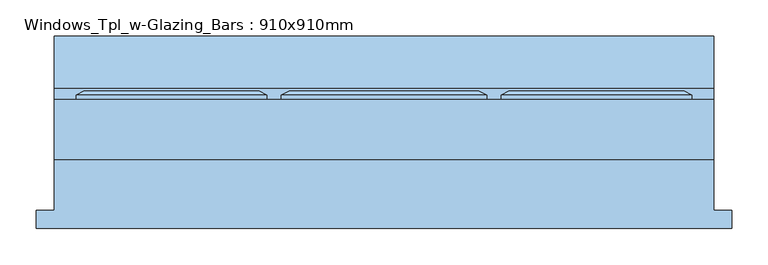
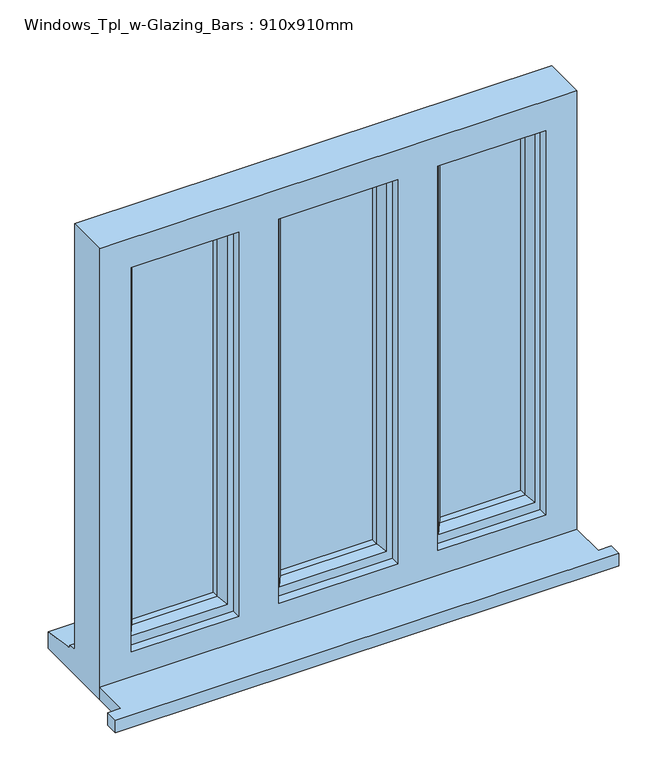
"""IFC4 building model written with IfcOpenShell, lengths in millimetres: window geometry, Windows_Tpl_w-Glazing_Bars : 910x910mm."""

from ifc_helpers import new_model, si_unit, frame, origin, place, context, project, spatial, polyline, outline, extrude, faceted_brep, source, transform, mapped, element, save


def windows_tpl_w_glazing_bars_910x910mm_9d987a72(model_context):
    return source(origin(), model_context, "Body", "SolidModel", [
        extrude(outline(polyline([(-716.6666667, -118.1434322), (-716.6666667, -93.1434322), (-691.6666667, -93.1434322), (-691.6666667, -22.9434322), (218.3333333, -22.9434322), (218.3333333, -93.1434322), (243.3333333, -93.1434322), (243.3333333, -118.1434322), (-716.6666667, -118.1434322)])), frame((0.0, 0.0, 1200.0), z_axis=(0.0, 0.0, 1.0), x_axis=(1.0, 0.0, 0.0)), (0.0, 0.0, 1.0), 25.0),
        faceted_brep([(-75.0, 60.0565678, 2080.0), (-75.0, 65.8300705, 2080.0), (-75.0, 65.8300705, 1253.0), (-75.0, 60.0565678, 1253.0), (-65.0, -4.9434322, 2070.0), (-65.0, 60.0565678, 2070.0), (-65.0, 60.0565678, 1263.0), (-65.0, -4.9434322, 1263.0), (-25.0, 9.5494677, 2030.0), (-35.1480377, -4.9434322, 2040.1480377), (-35.1480377, -4.9434322, 1292.8519623), (-25.0, 9.5494677, 1303.0), (-25.0, 24.0565678, 2030.0), (-25.0, 24.0565678, 1303.0), (-35.0, 48.0565678, 2040.0), (-35.0, 24.0565678, 2040.0), (-35.0, 24.0565678, 1293.0), (-35.0, 48.0565678, 1293.0), (-25.0, 65.8300705, 2030.0), (-25.0, 48.0565678, 2030.0), (-25.0, 48.0565678, 1303.0), (-25.0, 65.8300705, 1303.0), (-42.4457548, 71.6035732, 2047.4457548), (-42.4457548, 71.6035732, 1285.5542452), (-64.2153903, 71.6035732, 2069.2153903), (-64.2153903, 71.6035732, 1263.7846097), (188.3333333, 65.8300705, 1253.0), (188.3333333, 60.0565678, 1253.0), (178.3333333, 60.0565678, 1263.0), (178.3333333, -4.9434322, 1263.0), (148.4813711, -4.9434322, 1292.8519623), (138.3333333, 9.5494677, 1303.0), (138.3333333, 24.0565678, 1303.0), (148.3333333, 24.0565678, 1293.0), (148.3333333, 48.0565678, 1293.0), (138.3333333, 48.0565678, 1303.0), (138.3333333, 65.8300705, 1303.0), (155.7790881, 71.6035732, 1285.5542452), (177.5487236, 71.6035732, 1263.7846097), (188.3333333, 65.8300705, 2080.0), (188.3333333, 60.0565678, 2080.0), (178.3333333, 60.0565678, 2070.0), (178.3333333, -4.9434322, 2070.0), (148.4813711, -4.9434322, 2040.1480377), (138.3333333, 9.5494677, 2030.0), (138.3333333, 24.0565678, 2030.0), (148.3333333, 24.0565678, 2040.0), (148.3333333, 48.0565678, 2040.0), (138.3333333, 48.0565678, 2030.0), (138.3333333, 65.8300705, 2030.0), (155.7790881, 71.6035732, 2047.4457548), (177.5487236, 71.6035732, 2069.2153903)], [[[0, 1, 2, 3]], [[4, 5, 6, 7]], [[8, 9, 10, 11]], [[12, 8, 11, 13]], [[14, 15, 16, 17]], [[18, 19, 20, 21]], [[22, 18, 21, 23]], [[1, 24, 25, 2]], [[3, 2, 26, 27]], [[7, 6, 28, 29]], [[11, 10, 30, 31]], [[13, 11, 31, 32]], [[17, 16, 33, 34]], [[21, 20, 35, 36]], [[23, 21, 36, 37]], [[2, 25, 38, 26]], [[27, 26, 39, 40]], [[29, 28, 41, 42]], [[31, 30, 43, 44]], [[32, 31, 44, 45]], [[34, 33, 46, 47]], [[36, 35, 48, 49]], [[37, 36, 49, 50]], [[26, 38, 51, 39]], [[40, 39, 1, 0]], [[3, 27, 40, 0], [5, 41, 28, 6]], [[42, 41, 5, 4]], [[7, 29, 42, 4], [9, 43, 30, 10]], [[44, 43, 9, 8]], [[45, 44, 8, 12]], [[15, 46, 33, 16], [13, 32, 45, 12]], [[47, 46, 15, 14]], [[17, 34, 47, 14], [19, 48, 35, 20]], [[49, 48, 19, 18]], [[50, 49, 18, 22]], [[24, 51, 38, 25], [23, 37, 50, 22]], [[39, 51, 24, 1]]]),
        extrude(outline(polyline([(148.3333333, 24.0565678), (-35.1480377, 24.0565678), (-35.1480377, 48.0565678), (148.3333333, 48.0565678), (148.3333333, 24.0565678)])), frame((0.0, 0.0, 1293.0), z_axis=(0.0, 0.0, 1.0), x_axis=(1.0, 0.0, 0.0)), (0.0, 0.0, 1.0), 747.0),
        extrude(outline(polyline([(-135.0, 24.0565678), (-338.3333333, 24.0565678), (-338.3333333, 48.0565678), (-135.0, 48.0565678), (-135.0, 24.0565678)])), frame((0.0, 0.0, 1293.0), z_axis=(0.0, 0.0, 1.0), x_axis=(1.0, 0.0, 0.0)), (0.0, 0.0, 1.0), 747.0),
        extrude(outline(polyline([(-438.3333333, 24.0565678), (-621.6666667, 24.0565678), (-621.6666667, 48.0565678), (-438.3333333, 48.0565678), (-438.3333333, 24.0565678)])), frame((0.0, 0.0, 1293.0), z_axis=(0.0, 0.0, 1.0), x_axis=(1.0, 0.0, 0.0)), (0.0, 0.0, 1.0), 747.0),
        faceted_brep([(-398.3333333, 60.0565678, 2080.0), (-398.3333333, 65.8300705, 2080.0), (-661.6666667, 65.8300705, 2080.0), (-661.6666667, 60.0565678, 2080.0), (-408.3333333, -4.9434322, 2070.0), (-408.3333333, 60.0565678, 2070.0), (-651.6666667, 60.0565678, 2070.0), (-651.6666667, -4.9434322, 2070.0), (-448.3333333, 9.5494677, 2030.0), (-438.1852956, -4.9434322, 2040.1480377), (-621.8147044, -4.9434322, 2040.1480377), (-611.6666667, 9.5494677, 2030.0), (-448.3333333, 24.0565678, 2030.0), (-611.6666667, 24.0565678, 2030.0), (-438.3333333, 48.0565678, 2040.0), (-438.3333333, 24.0565678, 2040.0), (-621.6666667, 24.0565678, 2040.0), (-621.6666667, 48.0565678, 2040.0), (-448.3333333, 65.8300705, 2030.0), (-448.3333333, 48.0565678, 2030.0), (-611.6666667, 48.0565678, 2030.0), (-611.6666667, 65.8300705, 2030.0), (-430.8875785, 71.6035732, 2047.4457548), (-629.1124215, 71.6035732, 2047.4457548), (-409.117943, 71.6035732, 2069.2153903), (-650.882057, 71.6035732, 2069.2153903), (-661.6666667, 65.8300705, 1253.0), (-661.6666667, 60.0565678, 1253.0), (-651.6666667, 60.0565678, 1263.0), (-651.6666667, -4.9434322, 1263.0), (-621.8147044, -4.9434322, 1292.8519623), (-611.6666667, 9.5494677, 1303.0), (-611.6666667, 24.0565678, 1303.0), (-621.6666667, 24.0565678, 1293.0), (-621.6666667, 48.0565678, 1293.0), (-611.6666667, 48.0565678, 1303.0), (-611.6666667, 65.8300705, 1303.0), (-629.1124215, 71.6035732, 1285.5542452), (-650.882057, 71.6035732, 1263.7846097), (-398.3333333, 65.8300705, 1253.0), (-398.3333333, 60.0565678, 1253.0), (-408.3333333, 60.0565678, 1263.0), (-408.3333333, -4.9434322, 1263.0), (-438.1852956, -4.9434322, 1292.8519623), (-448.3333333, 9.5494677, 1303.0), (-448.3333333, 24.0565678, 1303.0), (-438.3333333, 24.0565678, 1293.0), (-438.3333333, 48.0565678, 1293.0), (-448.3333333, 48.0565678, 1303.0), (-448.3333333, 65.8300705, 1303.0), (-430.8875785, 71.6035732, 1285.5542452), (-409.117943, 71.6035732, 1263.7846097)], [[[0, 1, 2, 3]], [[4, 5, 6, 7]], [[8, 9, 10, 11]], [[12, 8, 11, 13]], [[14, 15, 16, 17]], [[18, 19, 20, 21]], [[22, 18, 21, 23]], [[1, 24, 25, 2]], [[3, 2, 26, 27]], [[7, 6, 28, 29]], [[11, 10, 30, 31]], [[13, 11, 31, 32]], [[17, 16, 33, 34]], [[21, 20, 35, 36]], [[23, 21, 36, 37]], [[2, 25, 38, 26]], [[27, 26, 39, 40]], [[0, 3, 27, 40], [41, 28, 6, 5]], [[29, 28, 41, 42]], [[4, 7, 29, 42], [43, 30, 10, 9]], [[31, 30, 43, 44]], [[32, 31, 44, 45]], [[46, 33, 16, 15], [12, 13, 32, 45]], [[34, 33, 46, 47]], [[14, 17, 34, 47], [48, 35, 20, 19]], [[36, 35, 48, 49]], [[37, 36, 49, 50]], [[51, 38, 25, 24], [22, 23, 37, 50]], [[26, 38, 51, 39]], [[40, 39, 1, 0]], [[42, 41, 5, 4]], [[44, 43, 9, 8]], [[45, 44, 8, 12]], [[47, 46, 15, 14]], [[49, 48, 19, 18]], [[50, 49, 18, 22]], [[39, 51, 24, 1]]]),
        extrude(outline(polyline([(-35.0, 40.0565678), (148.3333333, 40.0565678), (148.3333333, 32.0565678), (-35.0, 32.0565678), (-35.0, 40.0565678)])), frame((0.0, 0.0, 1656.5), z_axis=(0.0, 0.0, 1.0), x_axis=(1.0, 0.0, 0.0)), (0.0, 0.0, 1.0), 20.0),
        extrude(outline(polyline([(-621.6666667, 40.0565678), (-438.3333333, 40.0565678), (-438.3333333, 32.0565678), (-621.6666667, 32.0565678), (-621.6666667, 40.0565678)])), frame((0.0, 0.0, 1656.5), z_axis=(0.0, 0.0, 1.0), x_axis=(1.0, 0.0, 0.0)), (0.0, 0.0, 1.0), 20.0),
        extrude(outline(polyline([(-35.0, 40.0565678), (148.3333333, 40.0565678), (148.3333333, 32.0565678), (-35.0, 32.0565678), (-35.0, 40.0565678)])), frame((0.0, 0.0, 1838.25), z_axis=(0.0, 0.0, 1.0), x_axis=(1.0, 0.0, 0.0)), (0.0, 0.0, 1.0), 20.0),
        extrude(outline(polyline([(-35.0, 40.0565678), (148.3333333, 40.0565678), (148.3333333, 32.0565678), (-35.0, 32.0565678), (-35.0, 40.0565678)])), frame((0.0, 0.0, 1474.75), z_axis=(0.0, 0.0, 1.0), x_axis=(1.0, 0.0, 0.0)), (0.0, 0.0, 1.0), 20.0),
        extrude(outline(polyline([(-621.6666667, 40.0565678), (-438.3333333, 40.0565678), (-438.3333333, 32.0565678), (-621.6666667, 32.0565678), (-621.6666667, 40.0565678)])), frame((0.0, 0.0, 1838.25), z_axis=(0.0, 0.0, 1.0), x_axis=(1.0, 0.0, 0.0)), (0.0, 0.0, 1.0), 20.0),
        extrude(outline(polyline([(-621.6666667, 40.0565678), (-438.3333333, 40.0565678), (-438.3333333, 32.0565678), (-621.6666667, 32.0565678), (-621.6666667, 40.0565678)])), frame((0.0, 0.0, 1474.75), z_axis=(0.0, 0.0, 1.0), x_axis=(1.0, 0.0, 0.0)), (0.0, 0.0, 1.0), 20.0),
        extrude(outline(polyline([(-338.3333333, 40.0565678), (-135.0, 40.0565678), (-135.0, 32.0565678), (-338.3333333, 32.0565678), (-338.3333333, 40.0565678)])), frame((0.0, 0.0, 1656.5), z_axis=(0.0, 0.0, 1.0), x_axis=(1.0, 0.0, 0.0)), (0.0, 0.0, 1.0), 20.0),
        extrude(outline(polyline([(-338.3333333, 40.0565678), (-135.0, 40.0565678), (-135.0, 32.0565678), (-338.3333333, 32.0565678), (-338.3333333, 40.0565678)])), frame((0.0, 0.0, 1838.25), z_axis=(0.0, 0.0, 1.0), x_axis=(1.0, 0.0, 0.0)), (0.0, 0.0, 1.0), 20.0),
        extrude(outline(polyline([(-338.3333333, 40.0565678), (-135.0, 40.0565678), (-135.0, 32.0565678), (-338.3333333, 32.0565678), (-338.3333333, 40.0565678)])), frame((0.0, 0.0, 1474.75), z_axis=(0.0, 0.0, 1.0), x_axis=(1.0, 0.0, 0.0)), (0.0, 0.0, 1.0), 20.0),
        faceted_brep([(218.3333333, -22.9434322, 2110.0), (-691.6666667, -22.9434322, 2110.0), (-691.6666667, -22.9434322, 1200.0), (218.3333333, -22.9434322, 1200.0), (158.3333333, -22.9434322, 2050.0), (158.3333333, -22.9434322, 1275.0), (-47.0, -22.9434322, 1275.0), (-47.0, -22.9434322, 2050.0), (-123.0, -22.9434322, 2050.0), (-123.0, -22.9434322, 1275.0), (-350.3333333, -22.9434322, 1275.0), (-350.3333333, -22.9434322, 2050.0), (-426.3333333, -22.9434322, 2050.0), (-426.3333333, -22.9434322, 1275.0), (-631.6666667, -22.9434322, 1275.0), (-631.6666667, -22.9434322, 2050.0), (-691.6666667, 60.0565678, 2110.0), (-691.6666667, 60.0565678, 1251.0), (-691.6666667, 75.0565678, 1249.68767), (-691.6666667, 75.0565678, 1244.7449676), (-691.6666667, 147.5565678, 1233.8088847), (-691.6666667, 147.5565678, 1200.0), (218.3333333, 60.0565678, 2110.0), (218.3333333, 60.0565678, 1251.0), (-651.6666667, 60.0565678, 2070.0), (-651.6666667, 60.0565678, 1263.0), (-408.3333333, 60.0565678, 1263.0), (-408.3333333, 60.0565678, 2070.0), (-368.3333333, 60.0565678, 2070.0), (-368.3333333, 60.0565678, 1263.0), (-105.0, 60.0565678, 1263.0), (-105.0, 60.0565678, 2070.0), (-65.0, 60.0565678, 2070.0), (-65.0, 60.0565678, 1263.0), (178.3333333, 60.0565678, 1263.0), (178.3333333, 60.0565678, 2070.0), (-651.6666667, -4.9434322, 2070.0), (-651.6666667, -4.9434322, 1263.0), (-368.3333333, -4.9434322, 2070.0), (-105.0, -4.9434322, 2070.0), (-105.0, -4.9434322, 1263.0), (-368.3333333, -4.9434322, 1263.0), (-123.0, -4.9434322, 2050.0), (-350.3333333, -4.9434322, 2050.0), (-350.3333333, -4.9434322, 1275.0), (-123.0, -4.9434322, 1275.0), (-65.0, -4.9434322, 2070.0), (178.3333333, -4.9434322, 2070.0), (178.3333333, -4.9434322, 1263.0), (-65.0, -4.9434322, 1263.0), (158.3333333, -4.9434322, 2050.0), (-47.0, -4.9434322, 2050.0), (-47.0, -4.9434322, 1275.0), (158.3333333, -4.9434322, 1275.0), (-408.3333333, -4.9434322, 2070.0), (-408.3333333, -4.9434322, 1263.0), (-426.3333333, -4.9434322, 2050.0), (-631.6666667, -4.9434322, 2050.0), (-631.6666667, -4.9434322, 1275.0), (-426.3333333, -4.9434322, 1275.0), (218.3333333, 147.5565678, 1200.0), (218.3333333, 147.5565678, 1233.8088847), (218.3333333, 75.0565678, 1244.7449676), (218.3333333, 75.0565678, 1249.68767)], [[[0, 1, 2, 3], [4, 5, 6, 7], [8, 9, 10, 11], [12, 13, 14, 15]], [[2, 1, 16, 17, 18, 19, 20, 21]], [[17, 16, 22, 23], [24, 25, 26, 27], [28, 29, 30, 31], [32, 33, 34, 35]], [[25, 24, 36, 37]], [[38, 39, 40, 41], [42, 43, 44, 45]], [[46, 47, 48, 49], [50, 51, 52, 53]], [[36, 54, 55, 37], [56, 57, 58, 59]], [[57, 15, 14, 58]], [[1, 0, 22, 16]], [[36, 24, 27, 54]], [[35, 47, 46, 32]], [[38, 28, 31, 39]], [[15, 57, 56, 12]], [[50, 4, 7, 51]], [[11, 43, 42, 8]], [[23, 22, 0, 3, 60, 61, 62, 63]], [[35, 34, 48, 47]], [[4, 50, 53, 5]], [[43, 11, 10, 44]], [[12, 56, 59, 13]], [[27, 26, 55, 54]], [[29, 28, 38, 41]], [[31, 30, 40, 39]], [[33, 32, 46, 49]], [[51, 7, 6, 52]], [[8, 42, 45, 9]], [[60, 3, 2, 21]], [[61, 60, 21, 20]], [[62, 61, 20, 19]], [[63, 62, 19, 18]], [[23, 63, 18, 17]], [[26, 25, 37, 55]], [[34, 33, 49, 48]], [[41, 40, 30, 29]], [[6, 5, 53, 52]], [[45, 44, 10, 9]], [[59, 58, 14, 13]]]),
        faceted_brep([(-378.3333333, 60.0565678, 2080.0), (-378.3333333, 65.8300705, 2080.0), (-378.3333333, 65.8300705, 1253.0), (-378.3333333, 60.0565678, 1253.0), (-368.3333333, -4.9434322, 2070.0), (-368.3333333, 60.0565678, 2070.0), (-368.3333333, 60.0565678, 1263.0), (-368.3333333, -4.9434322, 1263.0), (-328.3333333, 9.5494677, 2030.0), (-338.4813711, -4.9434322, 2040.1480377), (-338.4813711, -4.9434322, 1292.8519623), (-328.3333333, 9.5494677, 1303.0), (-328.3333333, 24.0565678, 2030.0), (-328.3333333, 24.0565678, 1303.0), (-338.3333333, 48.0565678, 2040.0), (-338.3333333, 24.0565678, 2040.0), (-338.3333333, 24.0565678, 1293.0), (-338.3333333, 48.0565678, 1293.0), (-328.3333333, 65.8300705, 2030.0), (-328.3333333, 48.0565678, 2030.0), (-328.3333333, 48.0565678, 1303.0), (-328.3333333, 65.8300705, 1303.0), (-345.7790881, 71.6035732, 2047.4457548), (-345.7790881, 71.6035732, 1285.5542452), (-367.5487236, 71.6035732, 2069.2153903), (-367.5487236, 71.6035732, 1263.7846097), (-95.0, 65.8300705, 1253.0), (-95.0, 60.0565678, 1253.0), (-105.0, 60.0565678, 1263.0), (-105.0, -4.9434322, 1263.0), (-134.8519623, -4.9434322, 1292.8519623), (-145.0, 9.5494677, 1303.0), (-145.0, 24.0565678, 1303.0), (-135.0, 24.0565678, 1293.0), (-135.0, 48.0565678, 1293.0), (-145.0, 48.0565678, 1303.0), (-145.0, 65.8300705, 1303.0), (-127.5542452, 71.6035732, 1285.5542452), (-105.7846097, 71.6035732, 1263.7846097), (-95.0, 65.8300705, 2080.0), (-95.0, 60.0565678, 2080.0), (-105.0, 60.0565678, 2070.0), (-105.0, -4.9434322, 2070.0), (-134.8519623, -4.9434322, 2040.1480377), (-145.0, 9.5494677, 2030.0), (-145.0, 24.0565678, 2030.0), (-135.0, 24.0565678, 2040.0), (-135.0, 48.0565678, 2040.0), (-145.0, 48.0565678, 2030.0), (-145.0, 65.8300705, 2030.0), (-127.5542452, 71.6035732, 2047.4457548), (-105.7846097, 71.6035732, 2069.2153903)], [[[0, 1, 2, 3]], [[4, 5, 6, 7]], [[8, 9, 10, 11]], [[12, 8, 11, 13]], [[14, 15, 16, 17]], [[18, 19, 20, 21]], [[22, 18, 21, 23]], [[1, 24, 25, 2]], [[3, 2, 26, 27]], [[7, 6, 28, 29]], [[11, 10, 30, 31]], [[13, 11, 31, 32]], [[17, 16, 33, 34]], [[21, 20, 35, 36]], [[23, 21, 36, 37]], [[2, 25, 38, 26]], [[27, 26, 39, 40]], [[29, 28, 41, 42]], [[31, 30, 43, 44]], [[32, 31, 44, 45]], [[34, 33, 46, 47]], [[36, 35, 48, 49]], [[37, 36, 49, 50]], [[26, 38, 51, 39]], [[40, 39, 1, 0]], [[3, 27, 40, 0], [5, 41, 28, 6]], [[42, 41, 5, 4]], [[7, 29, 42, 4], [9, 43, 30, 10]], [[44, 43, 9, 8]], [[45, 44, 8, 12]], [[15, 46, 33, 16], [13, 32, 45, 12]], [[47, 46, 15, 14]], [[17, 34, 47, 14], [19, 48, 35, 20]], [[49, 48, 19, 18]], [[50, 49, 18, 22]], [[24, 51, 38, 25], [23, 37, 50, 22]], [[39, 51, 24, 1]]]),
    ])


if __name__ == "__main__":
    model = new_model("IFC4")
    model_context = context("Model", 3, world=origin())
    ifc_project = project(units=[si_unit("LENGTHUNIT", "METRE", prefix="MILLI")], contexts=[model_context])
    site = spatial("IfcSite", under=ifc_project)
    building = spatial("IfcBuilding", under=site)
    placement = place(None, origin())
    windows_tpl_w_glazing_bars_910x910mm_shape = windows_tpl_w_glazing_bars_910x910mm_9d987a72(model_context)
    element("IfcWindow", 1, ObjectType="Windows_Tpl_w-Glazing_Bars : 910x910mm", at=placement, inside=building, context=model_context, shape_type="MappedRepresentation", body=[
        mapped(windows_tpl_w_glazing_bars_910x910mm_shape, transform((0.0, 0.0, 0.0), x_axis=(1.0, 0.0, 0.0), y_axis=(0.0, 1.0, 0.0), z_axis=(0.0, 0.0, 1.0))),
    ])
    save(model, "model.ifc")

# Revit data of these elements
# Type "Windows_Tpl_w-Glazing_Bars : 910x910mm"
#   Type Mark = "18"
#   Operation = "TriplePanelVertical"
#   Construction Type Id = "GSP4R"
#   Manufacturer = "Revit"
#   Keynote = "L10"
#   Analytic Construction = "1/8 in Pilkington single glazing"
#   Length 1 = 24 mm
#   Wrap Layers (Ext) from Ext = 102.5 mm
#   Wrap Layers (Int) from Ext = 177.5 mm
#   Window Board Projection = 25 mm
#   Window Board Extension = 25 mm
#   Visual Light Transmittance = 0.9
#   Solar Heat Gain Coefficient = 0.78
#   Rough Width = 910 mm
#   Rough Height = 910 mm
#   Height = 910 mm
#   Width = 910 mm
#   Heat Transfer Coefficient (U) = 0.6496 BTU/(h·ft²·°F)
#   Glazing Thickness = 24 mm
#   Glazing Bar Thickness = 20 mm
#   FrameOffset - External = 50 mm
#   Frame Depth = 65 mm
#   Default Head Height = 2110 mm
#   Cill Depth = 87.5 mm
#   Cavity Closer Width = 50 mm
#   Cavity Closer Offset from Ext = 102.5 mm
#   Cavity Closer Depth = 85 mm
#   Vis - Glazing Bars = yes
#   Vis - Cavity Closers = yes
#   Define Thermal Properties by = 1
#   Material Trim = Window Frame
#   Material Glazing Bars = Window Frame
#   Material Glass = Glass
#   Material Frame = Window Frame
#   Wall Closure = (empty or 0)
# Element 1 (IfcWindow, "Windows_Tpl_w-Glazing_Bars : 910x910mm")
#   Materials on its faces: "Window Frame", "Glass"
# Materials
#   "Window Frame": colour RGB 249 249 249, transparency 0
#   "Glass": class "Glass", colour RGB 0 128 192, transparency 0.75, Description = "Soda Lime Glass", Cost = 0
